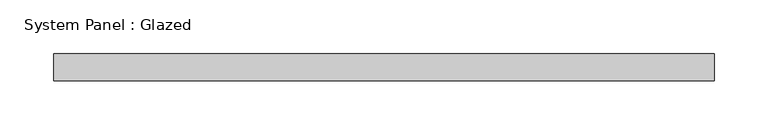
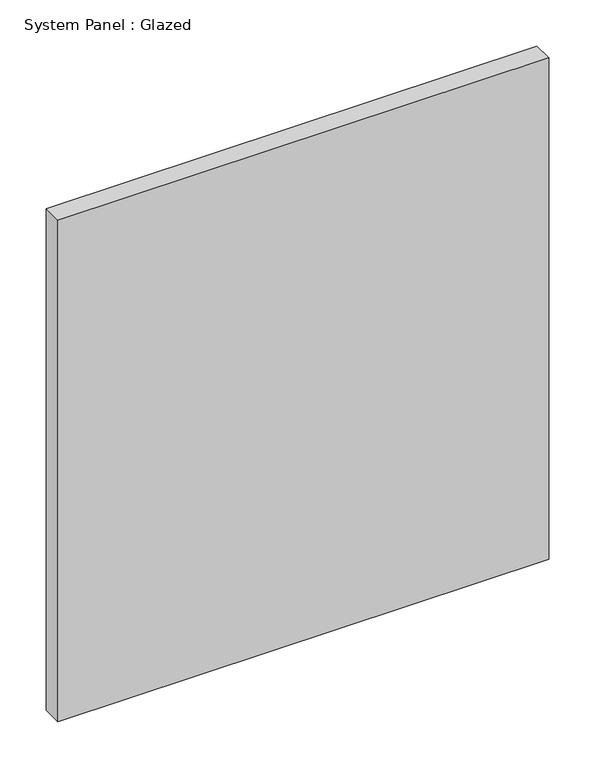
"""IFC4 building model written with IfcOpenShell, lengths in millimetres: plate geometry, System Panel : Glazed."""

from ifc_helpers import new_model, si_unit, origin, origin_with_axes, place, context, project, spatial, polyline, outline, extrude, source, transform, mapped, element, save


def system_panel_glazed_cd499e62(model_context):
    return source(origin(), model_context, "Body", "SweptSolid", [
        extrude(outline(polyline([(307.975, 19.05), (-307.975, 19.05), (-307.975, 44.45), (307.975, 44.45), (307.975, 19.05)])), origin_with_axes(), (0.0, 0.0, 1.0), 665.600254),
    ])


if __name__ == "__main__":
    model = new_model("IFC4")
    model_context = context("Model", 3, world=origin())
    ifc_project = project(units=[si_unit("LENGTHUNIT", "METRE", prefix="MILLI")], contexts=[model_context])
    site = spatial("IfcSite", under=ifc_project)
    building = spatial("IfcBuilding", under=site)
    placement = place(None, origin())
    system_panel_glazed_shape = system_panel_glazed_cd499e62(model_context)
    element("IfcPlate", 1, ObjectType="System Panel : Glazed", at=placement, inside=building, context=model_context, shape_type="MappedRepresentation", body=[
        mapped(system_panel_glazed_shape, transform((0.0, 0.0, 0.0), x_axis=(1.0, 0.0, 0.0), y_axis=(0.0, 1.0, 0.0), z_axis=(0.0, 0.0, 1.0))),
    ])
    save(model, "model.ifc")

# Revit data of these elements
# Type "System Panel : Glazed"
#   Construction Type Id = "GSP4R"
#   Analytic Construction = "1/8 in Pilkington single glazing"
#   Visual Light Transmittance = 0.9
#   Solar Heat Gain Coefficient = 0.86
#   Heat Transfer Coefficient (U) = 1.18115 BTU/(h·ft²·°F)
#   Define Thermal Properties by = 1
# Element 1 (IfcPlate, "System Panel : Glazed")
#   Materials on its faces: "Glass"
# Materials
#   "Glass": class "Glass", colour RGB 0 128 192, transparency 0.75, Description = "Soda Lime Glass", Cost = 0
